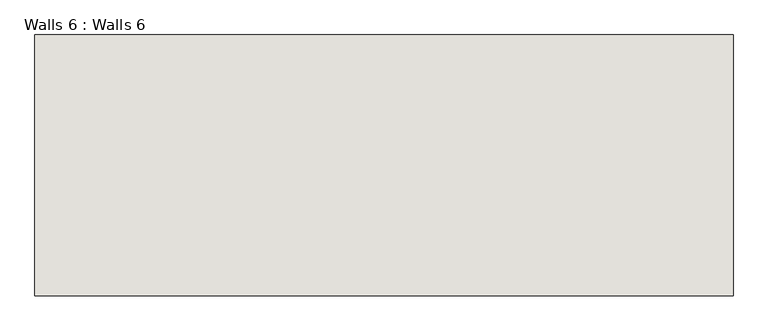
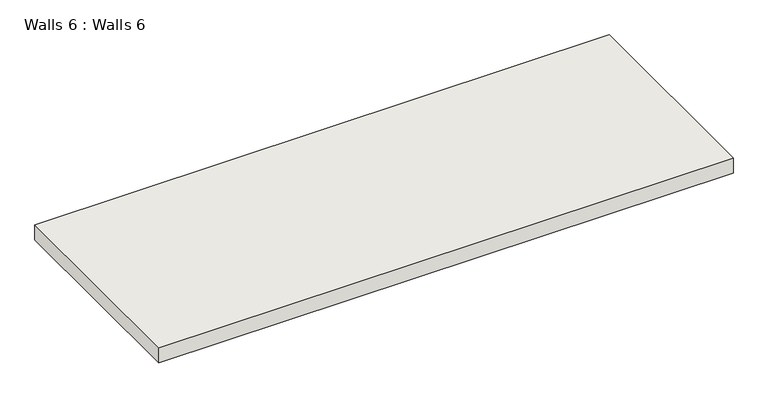
"""IFC4 building model written with IfcOpenShell, lengths in millimetres: wall geometry, Walls 6 : Walls 6."""

from ifc_helpers import new_model, si_unit, frame, origin, place, context, project, spatial, polyline, outline, extrude, source, transform, mapped, element, save


def walls_6_walls_6_d361cd03(model_context):
    return source(origin(), model_context, "Body", "SweptSolid", [
        extrude(outline(polyline([(-16232.0897324, -4103.7180898), (-16232.0897324, -3390.9180898), (-14325.4897324, -3390.9180898), (-14325.4897324, -4103.7180898), (-16232.0897324, -4103.7180898)])), frame((0.0, 0.0, 2762.6009455), z_axis=(0.0, 0.0, 1.0), x_axis=(1.0, 0.0, 0.0)), (0.0, 0.0, 1.0), 52.693252),
    ])


if __name__ == "__main__":
    model = new_model("IFC4")
    model_context = context("Model", 3, world=origin())
    ifc_project = project(units=[si_unit("LENGTHUNIT", "METRE", prefix="MILLI")], contexts=[model_context])
    site = spatial("IfcSite", under=ifc_project)
    building = spatial("IfcBuilding", under=site)
    placement = place(None, origin())
    walls_6_walls_6_shape = walls_6_walls_6_d361cd03(model_context)
    element("IfcWall", 1, ObjectType="Walls 6 : Walls 6", at=placement, inside=building, context=model_context, shape_type="MappedRepresentation", body=[
        mapped(walls_6_walls_6_shape, transform((0.0, 0.0, 0.0), x_axis=(1.0, 0.0, 0.0), y_axis=(0.0, 1.0, 0.0), z_axis=(0.0, 0.0, 1.0))),
    ])
    save(model, "model.ifc")

# Revit data of these elements
# Element 1 (IfcWall, "Walls 6 : Walls 6")
#   Materials on its faces: "Default Wall"
# Materials
#   "Default Wall": colour RGB 80 80 80, transparency 0
